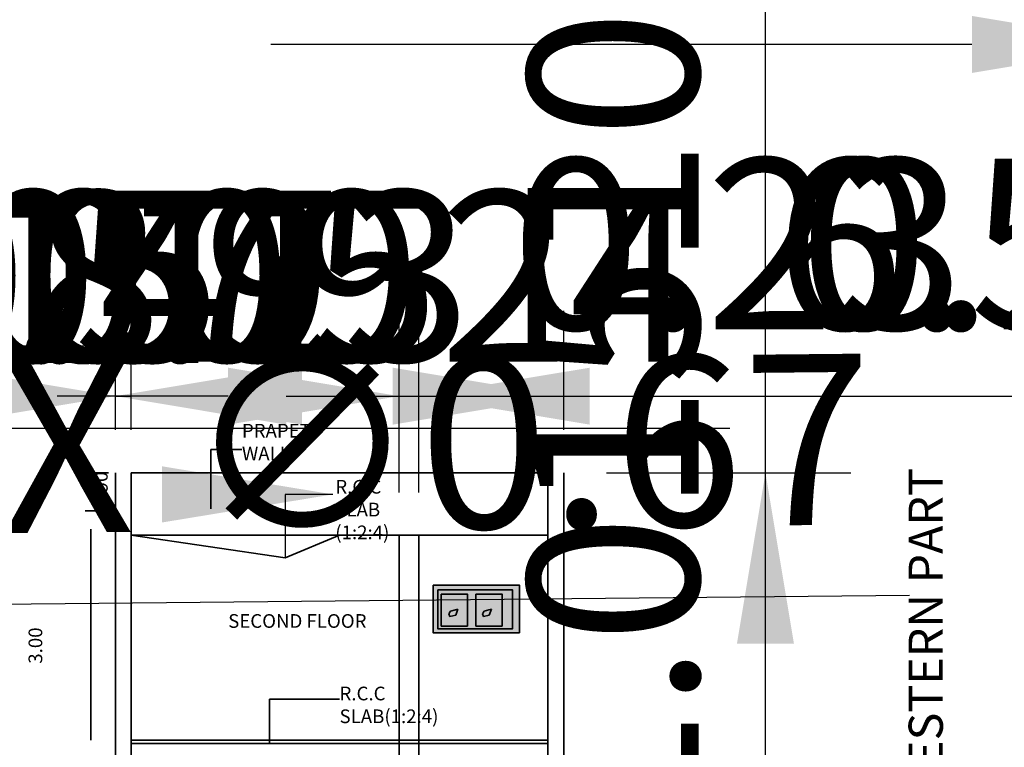
# Model space of a CAD drawing. Units: metres. Extents: x 782 to 1487, y 1262 to 7446.
# Tile 21 of 25: x 801.93 to 816.33, y 1326.35 to 1336.99. Entities that reach past the tile are written whole.
import ezdxf

# ---------------------------------------------------------------- set-up
doc = ezdxf.new("R2010")
doc.units = ezdxf.units.M
for name, color, linetype, lineweight in [('A-ANNO-DIMS', 2, 'Continuous', 18), ('A-ANNO-TEXT', 3, 'Continuous', 18), ('A-SECT', 7, 'Continuous', 35), ('A-SECT-PATT', 9, 'Continuous', 13)]:
    doc.layers.add(name, color=color, linetype=linetype, lineweight=lineweight)
doc.styles.get("Standard").update_dxf_attribs({"font": 'arial.ttf'})
doc.dimstyles.new('ISO-25', dxfattribs={"dimtxt": 2.5, "dimasz": 2.5, "dimexe": 1.25, "dimexo": 0.625, "dimtad": 1, "dimtxsty": 'Standard', "dimcen": 2.5, "dimadec": 0, "dimazin": 0, "dimtfac": 1, "dimtmove": 0, "dimatfit": 3, "dimfxl": 1, "dimarcsym": 0})

# ---------------------------------------------------------------- blocks, each defined once
blk = doc.blocks.new('*D12')
at = {"layer": 'A-ANNO-DIMS', "color": 0, "lineweight": -2, "transparency": 16777216}
for p, q in [((818.357, 1335.252), (818.357, 1337.877)), ((823.837, 1335.252), (823.837, 1337.877)), ((815.857, 1336.627), (805.608, 1336.627)), ((823.837, 1336.627), (818.357, 1336.627)), ((826.337, 1336.627), (828.837, 1336.627))]:
    blk.add_line(p, q, dxfattribs=at)
at = {"layer": 'A-ANNO-DIMS', "color": 0, "transparency": 16777216}
for points in [[(815.857, 1337.044), (815.857, 1336.21), (818.357, 1336.627)], [(826.337, 1337.044), (826.337, 1336.21), (823.837, 1336.627)]]:
    blk.add_solid(points, dxfattribs=at)
at = {"layer": 'Defpoints', "color": 0, "transparency": 16777216}
for p in [(818.357, 1336.627), (818.357, 1334.627), (823.837, 1334.627)]:
    blk.add_point(p, dxfattribs=at)
at = {"layer": 'A-ANNO-DIMS', "color": 0, "transparency": 16777216, "insert": (809.482, 1338.754), "char_height": 2.5, "width": 6.51678, "attachment_point": 5}
blk.add_mtext('5,48', dxfattribs=at)
blk = doc.blocks.new('*D116')
at = {"layer": 'A-ANNO-DIMS', "color": 0, "lineweight": -2, "transparency": 16777216}
for p, q in [((791.782, 1330.988), (791.782, 1332.263)), ((792.923, 1329.614), (792.923, 1332.263)), ((789.282, 1331.013), (786.782, 1331.013)), ((791.782, 1331.013), (792.923, 1331.013)), ((795.423, 1331.013), (805.421, 1331.013))]:
    blk.add_line(p, q, dxfattribs=at)
at = {"layer": 'A-ANNO-DIMS', "color": 0, "transparency": 16777216}
for points in [[(789.282, 1331.43), (789.282, 1330.597), (791.782, 1331.013)], [(795.423, 1331.43), (795.423, 1330.597), (792.923, 1331.013)]]:
    blk.add_solid(points, dxfattribs=at)
at = {"layer": 'Defpoints', "color": 0, "transparency": 16777216}
for p in [(792.923, 1331.013), (791.782, 1330.363), (792.923, 1328.989)]:
    blk.add_point(p, dxfattribs=at)
at = {"layer": 'A-ANNO-DIMS', "color": 0, "transparency": 16777216, "insert": (801.672, 1332.894), "char_height": 2.5, "attachment_point": 5}
blk.add_mtext('1.14', dxfattribs=at)
blk = doc.blocks.new('*D117')
at = {"layer": 'A-ANNO-DIMS', "color": 0, "lineweight": -2, "transparency": 16777216}
for p, q in [((792.923, 1329.614), (792.923, 1332.263)), ((793.726, 1327.207), (793.726, 1332.263)), ((790.423, 1331.013), (787.923, 1331.013)), ((792.923, 1331.013), (793.726, 1331.013)), ((796.226, 1331.013), (806.461, 1331.013))]:
    blk.add_line(p, q, dxfattribs=at)
at = {"layer": 'A-ANNO-DIMS', "color": 0, "transparency": 16777216}
for points in [[(790.423, 1331.43), (790.423, 1330.597), (792.923, 1331.013)], [(796.226, 1331.43), (796.226, 1330.597), (793.726, 1331.013)]]:
    blk.add_solid(points, dxfattribs=at)
at = {"layer": 'Defpoints', "color": 0, "transparency": 16777216}
for p in [(793.726, 1331.013), (792.923, 1328.989), (793.726, 1326.582)]:
    blk.add_point(p, dxfattribs=at)
at = {"layer": 'A-ANNO-DIMS', "color": 0, "transparency": 16777216, "insert": (802.594, 1332.915), "char_height": 2.5, "attachment_point": 5}
blk.add_mtext('0.80', dxfattribs=at)
blk = doc.blocks.new('*D118')
at = {"layer": 'A-ANNO-DIMS', "color": 0, "lineweight": -2, "transparency": 16777216}
for p, q in [((793.726, 1327.207), (793.726, 1332.263)), ((794.32, 1327.207), (794.32, 1332.263)), ((791.226, 1331.013), (788.726, 1331.013)), ((793.726, 1331.013), (794.32, 1331.013)), ((796.82, 1331.013), (807.069, 1331.013))]:
    blk.add_line(p, q, dxfattribs=at)
at = {"layer": 'A-ANNO-DIMS', "color": 0, "transparency": 16777216}
for points in [[(791.226, 1331.43), (791.226, 1330.597), (793.726, 1331.013)], [(796.82, 1331.43), (796.82, 1330.597), (794.32, 1331.013)]]:
    blk.add_solid(points, dxfattribs=at)
at = {"layer": 'Defpoints', "color": 0, "transparency": 16777216}
for p in [(794.32, 1331.013), (793.726, 1326.582), (794.32, 1326.582)]:
    blk.add_point(p, dxfattribs=at)
at = {"layer": 'A-ANNO-DIMS', "color": 0, "transparency": 16777216, "insert": (803.194, 1332.915), "char_height": 2.5, "attachment_point": 5}
blk.add_mtext('0.59', dxfattribs=at)
blk = doc.blocks.new('*D119')
at = {"layer": 'A-ANNO-DIMS', "color": 0, "lineweight": -2, "transparency": 16777216}
for p, q in [((794.32, 1327.207), (794.32, 1332.263)), ((794.83, 1330.074), (794.83, 1332.263)), ((791.82, 1331.013), (789.32, 1331.013)), ((794.32, 1331.013), (794.83, 1331.013)), ((797.33, 1331.013), (807.091, 1331.013))]:
    blk.add_line(p, q, dxfattribs=at)
at = {"layer": 'A-ANNO-DIMS', "color": 0, "transparency": 16777216}
for points in [[(791.82, 1331.43), (791.82, 1330.597), (794.32, 1331.013)], [(797.33, 1331.43), (797.33, 1330.597), (794.83, 1331.013)]]:
    blk.add_solid(points, dxfattribs=at)
at = {"layer": 'Defpoints', "color": 0, "transparency": 16777216}
for p in [(794.83, 1331.013), (794.83, 1329.449), (794.32, 1326.582)]:
    blk.add_point(p, dxfattribs=at)
at = {"layer": 'A-ANNO-DIMS', "color": 0, "transparency": 16777216, "insert": (803.46, 1332.915), "char_height": 2.5, "attachment_point": 5}
blk.add_mtext('0.51', dxfattribs=at)
blk = doc.blocks.new('*D120')
at = {"layer": 'A-ANNO-DIMS', "color": 0, "lineweight": -2, "transparency": 16777216}
for p, q in [((794.83, 1330.074), (794.83, 1332.263)), ((795.62, 1329.519), (795.62, 1332.263)), ((792.33, 1331.013), (789.83, 1331.013)), ((794.83, 1331.013), (795.62, 1331.013)), ((798.12, 1331.013), (808.369, 1331.013))]:
    blk.add_line(p, q, dxfattribs=at)
at = {"layer": 'A-ANNO-DIMS', "color": 0, "transparency": 16777216}
for points in [[(792.33, 1331.43), (792.33, 1330.597), (794.83, 1331.013)], [(798.12, 1331.43), (798.12, 1330.597), (795.62, 1331.013)]]:
    blk.add_solid(points, dxfattribs=at)
at = {"layer": 'Defpoints', "color": 0, "transparency": 16777216}
for p in [(795.62, 1331.013), (794.83, 1329.449), (795.62, 1328.894)]:
    blk.add_point(p, dxfattribs=at)
at = {"layer": 'A-ANNO-DIMS', "color": 0, "transparency": 16777216, "insert": (804.495, 1332.915), "char_height": 2.5, "attachment_point": 5}
blk.add_mtext('0.79', dxfattribs=at)
blk = doc.blocks.new('*D121')
at = {"layer": 'A-ANNO-DIMS', "color": 0, "lineweight": -2, "transparency": 16777216}
for p, q in [((795.62, 1329.519), (795.62, 1332.263)), ((796.354, 1329.519), (796.354, 1332.263)), ((793.12, 1331.013), (790.62, 1331.013)), ((795.62, 1331.013), (796.354, 1331.013)), ((798.854, 1331.013), (809.098, 1331.013))]:
    blk.add_line(p, q, dxfattribs=at)
at = {"layer": 'A-ANNO-DIMS', "color": 0, "transparency": 16777216}
for points in [[(793.12, 1331.43), (793.12, 1330.597), (795.62, 1331.013)], [(798.854, 1331.43), (798.854, 1330.597), (796.354, 1331.013)]]:
    blk.add_solid(points, dxfattribs=at)
at = {"layer": 'Defpoints', "color": 0, "transparency": 16777216}
for p in [(796.354, 1331.013), (795.62, 1328.894), (796.354, 1328.894)]:
    blk.add_point(p, dxfattribs=at)
at = {"layer": 'A-ANNO-DIMS', "color": 0, "transparency": 16777216, "insert": (805.226, 1332.916), "char_height": 2.5, "attachment_point": 5}
blk.add_mtext('0.73', dxfattribs=at)
blk = doc.blocks.new('*D122')
at = {"layer": 'A-ANNO-DIMS', "color": 0, "lineweight": -2, "transparency": 16777216}
for p, q in [((796.354, 1329.519), (796.354, 1332.263)), ((797.878, 1330.988), (797.878, 1332.263)), ((793.854, 1331.013), (791.354, 1331.013)), ((796.354, 1331.013), (797.878, 1331.013)), ((800.378, 1331.013), (812.318, 1331.013))]:
    blk.add_line(p, q, dxfattribs=at)
at = {"layer": 'A-ANNO-DIMS', "color": 0, "transparency": 16777216}
for points in [[(793.854, 1331.43), (793.854, 1330.597), (796.354, 1331.013)], [(800.378, 1331.43), (800.378, 1330.597), (797.878, 1331.013)]]:
    blk.add_solid(points, dxfattribs=at)
at = {"layer": 'Defpoints', "color": 0, "transparency": 16777216}
for p in [(797.878, 1331.013), (797.878, 1330.363), (796.354, 1328.894)]:
    blk.add_point(p, dxfattribs=at)
at = {"layer": 'A-ANNO-DIMS', "color": 0, "transparency": 16777216, "insert": (807.598, 1332.915), "char_height": 2.5, "attachment_point": 5}
blk.add_mtext('1.524', dxfattribs=at)
blk = doc.blocks.new('*D137')
at = {"layer": 'A-ANNO-DIMS', "color": 0, "lineweight": -2, "transparency": 16777216}
for p, q in [((803.332, 1330.988), (803.332, 1332.733)), ((809.888, 1330.988), (809.888, 1332.733)), ((805.832, 1331.483), (807.388, 1331.483)), ((809.888, 1331.483), (822.086, 1331.483))]:
    blk.add_line(p, q, dxfattribs=at)
at = {"layer": 'A-ANNO-DIMS', "color": 0, "transparency": 16777216}
for points in [[(805.832, 1331.899), (805.832, 1331.066), (803.332, 1331.483)], [(807.388, 1331.899), (807.388, 1331.066), (809.888, 1331.483)]]:
    blk.add_solid(points, dxfattribs=at)
at = {"layer": 'Defpoints', "color": 0, "transparency": 16777216}
for p in [(809.888, 1331.483), (803.332, 1330.363), (809.888, 1330.363)]:
    blk.add_point(p, dxfattribs=at)
at = {"layer": 'A-ANNO-DIMS', "color": 0, "transparency": 16777216, "insert": (817.237, 1333.384), "char_height": 2.5, "attachment_point": 5}
blk.add_mtext('6.556', dxfattribs=at)
blk = doc.blocks.new('*D138')
at = {"layer": 'A-ANNO-DIMS', "color": 0, "lineweight": -2, "transparency": 16777216}
for p, q in [((803.332, 1330.988), (803.332, 1332.733)), ((803.562, 1330.988), (803.562, 1332.733)), ((800.832, 1331.483), (798.332, 1331.483)), ((803.332, 1331.483), (803.562, 1331.483)), ((806.062, 1331.483), (816.306, 1331.483))]:
    blk.add_line(p, q, dxfattribs=at)
at = {"layer": 'A-ANNO-DIMS', "color": 0, "transparency": 16777216}
for points in [[(800.832, 1331.899), (800.832, 1331.066), (803.332, 1331.483)], [(806.062, 1331.899), (806.062, 1331.066), (803.562, 1331.483)]]:
    blk.add_solid(points, dxfattribs=at)
at = {"layer": 'Defpoints', "color": 0, "transparency": 16777216}
for p in [(803.562, 1331.483), (803.332, 1330.363), (803.562, 1330.363)]:
    blk.add_point(p, dxfattribs=at)
at = {"layer": 'A-ANNO-DIMS', "color": 0, "transparency": 16777216, "insert": (812.434, 1333.385), "char_height": 2.5, "attachment_point": 5}
blk.add_mtext('0.23', dxfattribs=at)
blk = doc.blocks.new('*D139')
at = {"layer": 'A-ANNO-DIMS', "color": 0, "lineweight": -2, "transparency": 16777216}
for p, q in [((807.481, 1330.074), (807.481, 1332.733)), ((807.769, 1330.074), (807.769, 1332.733)), ((804.981, 1331.483), (802.481, 1331.483)), ((807.481, 1331.483), (807.769, 1331.483)), ((810.269, 1331.483), (820.518, 1331.483))]:
    blk.add_line(p, q, dxfattribs=at)
at = {"layer": 'A-ANNO-DIMS', "color": 0, "transparency": 16777216}
for points in [[(804.981, 1331.899), (804.981, 1331.066), (807.481, 1331.483)], [(810.269, 1331.899), (810.269, 1331.066), (807.769, 1331.483)]]:
    blk.add_solid(points, dxfattribs=at)
at = {"layer": 'Defpoints', "color": 0, "transparency": 16777216}
for p in [(807.769, 1331.483), (807.481, 1329.449), (807.769, 1329.449)]:
    blk.add_point(p, dxfattribs=at)
at = {"layer": 'A-ANNO-DIMS', "color": 0, "transparency": 16777216, "insert": (816.644, 1333.384), "char_height": 2.5, "attachment_point": 5}
blk.add_mtext('0.29', dxfattribs=at)
blk = doc.blocks.new('*D145')
at = {"layer": 'A-ANNO-DIMS', "color": 0, "lineweight": -2, "transparency": 16777216}
for p, q in [((812.839, 1322.045), (812.839, 1334.015)), ((811.308, 1319.545), (814.089, 1319.545)), ((812.839, 1318.53), (812.839, 1319.545)), ((811.308, 1318.53), (814.089, 1318.53)), ((812.839, 1316.03), (812.839, 1313.53))]:
    blk.add_line(p, q, dxfattribs=at)
at = {"layer": 'A-ANNO-DIMS', "color": 0, "transparency": 16777216}
for points in [[(812.422, 1322.045), (813.255, 1322.045), (812.839, 1319.545)], [(812.422, 1316.03), (813.255, 1316.03), (812.839, 1318.53)]]:
    blk.add_solid(points, dxfattribs=at)
at = {"layer": 'Defpoints', "color": 0, "transparency": 16777216}
for p in [(810.683, 1319.545), (812.839, 1319.545), (810.683, 1318.53)]:
    blk.add_point(p, dxfattribs=at)
at = {"layer": 'A-ANNO-DIMS', "color": 0, "transparency": 16777216, "insert": (810.937, 1329.28), "char_height": 2.5, "attachment_point": 5, "rotation": 90}
blk.add_mtext('1.015', dxfattribs=at)
blk = doc.blocks.new('*D146')
at = {"layer": 'A-ANNO-DIMS', "color": 0, "lineweight": -2, "transparency": 16777216}
for p, q in [((812.839, 1330.363), (812.839, 1344.262)), ((810.513, 1330.363), (814.089, 1330.363)), ((812.839, 1322.045), (812.839, 1327.863)), ((810.513, 1319.545), (814.089, 1319.545))]:
    blk.add_line(p, q, dxfattribs=at)
at = {"layer": 'A-ANNO-DIMS', "color": 0, "transparency": 16777216}
for points in [[(812.422, 1327.863), (813.255, 1327.863), (812.839, 1330.363)], [(812.422, 1322.045), (813.255, 1322.045), (812.839, 1319.545)]]:
    blk.add_solid(points, dxfattribs=at)
at = {"layer": 'Defpoints', "color": 0, "transparency": 16777216}
for p in [(809.888, 1330.363), (812.839, 1330.363), (809.888, 1319.545)]:
    blk.add_point(p, dxfattribs=at)
at = {"layer": 'A-ANNO-DIMS', "color": 0, "transparency": 16777216, "insert": (810.937, 1338.563), "char_height": 2.5, "attachment_point": 5, "rotation": 90}
blk.add_mtext('10.818', dxfattribs=at)
blk = doc.blocks.new('*D170')
at = {"layer": 'A-ANNO-DIMS', "color": 0, "lineweight": -2, "transparency": 16777216}
for p, q in [((814.947, 1328.566), (796.747, 1328.385)), ((791.077, 1328.328), (788.578, 1328.304)), ((793.577, 1328.353), (794.248, 1328.36))]:
    blk.add_line(p, q, dxfattribs=at)
at = {"layer": 'A-ANNO-DIMS', "color": 0, "transparency": 16777216}
for points in [[(791.073, 1328.745), (791.082, 1327.912), (793.577, 1328.353)], [(796.743, 1328.802), (796.752, 1327.968), (794.248, 1328.36)]]:
    blk.add_solid(points, dxfattribs=at)
at = {"layer": 'Defpoints', "color": 0, "transparency": 16777216}
for p in [(793.577, 1328.353), (794.248, 1328.36)]:
    blk.add_point(p, dxfattribs=at)
at = {"layer": 'A-ANNO-DIMS', "color": 0, "transparency": 16777216, "insert": (807.078, 1330.459), "char_height": 2.5, "attachment_point": 5, "rotation": 0.5708}
blk.add_mtext('3X ∅0.67', dxfattribs=at)

msp = doc.modelspace()

# ---------------------------------------------------------------- hatches: boundary and pattern name
at = {"layer": 'A-SECT-PATT'}
h = msp.add_hatch(color=256, dxfattribs=at)
h.dxf.hatch_style = 1
h.paths.add_polyline_path([(809.2411, 1328.7199), (807.9777, 1328.7199), (807.9777, 1328.0213), (809.2411, 1328.0213)])
h.paths.add_polyline_path([(809.1376, 1328.0792), (808.0486, 1328.0792), (808.0486, 1328.6511), (809.1376, 1328.6511)], flags=16)
h.paths.add_polyline_path([(808.9875, 1328.1205), (808.6043, 1328.1205), (808.6043, 1328.5874), (808.9875, 1328.5874)], flags=0)
h.paths.add_polyline_path([(808.4803, 1328.1205), (808.0971, 1328.1205), (808.0971, 1328.5874), (808.4803, 1328.5874)], flags=0)
h = msp.add_hatch(color=256, dxfattribs=at)
h.dxf.hatch_style = 1
h.paths.add_polyline_path([(809.1376, 1328.6511), (808.0486, 1328.6511), (808.0486, 1328.0792), (809.1376, 1328.0792)])
h.paths.add_polyline_path([(808.4803, 1328.5874), (808.4803, 1328.1205), (808.0971, 1328.1205), (808.0971, 1328.5874)], flags=16)
h.paths.add_polyline_path([(808.3426, 1328.3672), (808.3106, 1328.2799), (808.224, 1328.2583), (808.2108, 1328.2968), (808.2343, 1328.3373), (808.3059, 1328.357)], flags=0)
h.paths.add_polyline_path([(808.6043, 1328.5874), (808.9875, 1328.5874), (808.9875, 1328.1205), (808.6043, 1328.1205)], flags=16)
h.paths.add_polyline_path([(808.7238, 1328.3373), (808.7953, 1328.357), (808.8321, 1328.3672), (808.8, 1328.2799), (808.7134, 1328.2583), (808.7002, 1328.2968)], flags=0)
h = msp.add_hatch(color=256, dxfattribs=at)
h.dxf.hatch_style = 1
h.paths.add_polyline_path([(808.4803, 1328.5874), (808.0971, 1328.5874), (808.0971, 1328.1205), (808.4803, 1328.1205)])
h.paths.add_polyline_path([(808.3106, 1328.2799), (808.224, 1328.2583), (808.2108, 1328.2968), (808.2343, 1328.3373), (808.3059, 1328.357), (808.3426, 1328.3672)], flags=16)
h.paths.add_polyline_path([(808.9875, 1328.5874), (808.6043, 1328.5874), (808.6043, 1328.1205), (808.9875, 1328.1205)])
h.paths.add_polyline_path([(808.7238, 1328.3373), (808.7953, 1328.357), (808.8321, 1328.3672), (808.8, 1328.2799), (808.7134, 1328.2583), (808.7002, 1328.2968)], flags=16)
h = msp.add_hatch(color=256, dxfattribs=at)
h.dxf.hatch_style = 1
h.paths.add_polyline_path([(808.3426, 1328.3672), (808.3059, 1328.357), (808.2343, 1328.3373), (808.2108, 1328.2968), (808.224, 1328.2583), (808.3106, 1328.2799)])
h.paths.add_polyline_path([(808.8321, 1328.3672), (808.7953, 1328.357), (808.7238, 1328.3373), (808.7002, 1328.2968), (808.7134, 1328.2583), (808.8, 1328.2799)])

# ---------------------------------------------------------------- linework, layer by layer
at = {"layer": 'A-SECT'}
for p, q in [((805.1827, 1330.7028), (804.7268, 1330.7028)), ((804.7268, 1330.7028), (804.7268, 1329.8359)), ((802.8929, 1330.3635), (803.233, 1330.3635)), ((803.3321, 1320.4591), (803.3321, 1330.3635)), ((803.5621, 1330.3635), (809.6581, 1330.3635)), ((803.5621, 1320.4591), (803.5621, 1330.3635)), ((809.6581, 1320.4591), (809.6581, 1330.3635)), ((809.8881, 1320.4591), (809.8881, 1330.3635)), ((803.2609, 1329.8066), (802.8929, 1329.8066)), ((802.9742, 1326.4523), (802.9742, 1329.5361)), ((803.5621, 1329.4495), (809.6581, 1329.4495)), ((805.8175, 1329.1172), (803.5621, 1329.4495)), ((805.8175, 1329.1172), (806.6101, 1329.4495)), ((806.6101, 1329.4495), (805.8175, 1329.1172)), ((807.4812, 1320.4591), (807.4812, 1329.4495)), ((807.7695, 1320.4591), (807.7695, 1329.4495)), ((808.2108, 1328.2968), (808.2343, 1328.3373)), ((808.224, 1328.2583), (808.2108, 1328.2968)), ((808.3106, 1328.2799), (808.224, 1328.2583)), ((808.2343, 1328.3373), (808.3059, 1328.357)), ((808.3059, 1328.357), (808.3426, 1328.3672)), ((808.3426, 1328.3672), (808.3106, 1328.2799)), ((808.7002, 1328.2968), (808.7238, 1328.3373)), ((808.7134, 1328.2583), (808.7002, 1328.2968)), ((808.8, 1328.2799), (808.7134, 1328.2583)), ((808.7238, 1328.3373), (808.7953, 1328.357)), ((808.7953, 1328.357), (808.8321, 1328.3672)), ((808.8321, 1328.3672), (808.8, 1328.2799)), ((805.5843, 1326.4015), (805.5843, 1327.0483)), ((805.5843, 1327.0483), (806.6101, 1327.0483)), ((803.5621, 1326.4523), (809.6581, 1326.4523)), ((803.5621, 1326.4015), (809.6581, 1326.4015)), ((806.6101, 1326.4015), (805.5843, 1326.4015))]:
    msp.add_line(p, q, dxfattribs=at)
for points in [[(807.9777, 1328.7199), (809.2411, 1328.7199), (809.2411, 1328.0213), (807.9777, 1328.0213)], [(808.0486, 1328.6511), (809.1376, 1328.6511), (809.1376, 1328.0792), (808.0486, 1328.0792)], [(808.0971, 1328.5874), (808.4803, 1328.5874), (808.4803, 1328.1205), (808.0971, 1328.1205)], [(808.6043, 1328.5874), (808.9875, 1328.5874), (808.9875, 1328.1205), (808.6043, 1328.1205)]]:
    msp.add_lwpolyline(points, close=True, dxfattribs=at)

# ---------------------------------------------------------------- texts
at = {"layer": 'A-ANNO-TEXT', "char_height": 0.2, "attachment_point": 1}
for s, width, insert in [('\\P\\PPRAPET WALL ', 1.427343, (805.1827, 1331.7444)), ('\\P\\PR.C.C SLAB (1:2:4)', 1.016389, (806.5485, 1330.9238)), ('\\PSECOND FLOOR', 3.104755, (804.9819, 1328.6275)), ('\\PR.C.C SLAB(1:2:4)', 1.857201, (806.6101, 1327.5668))]:
    msp.add_mtext_dynamic_manual_height_columns(s, width=width, gutter_width=12.5, heights=[0], dxfattribs=dict(at, insert=insert))
at = {"layer": 'A-ANNO-TEXT', "attachment_point": 1, "rotation": 90}
for s, width, insert, char_height in [('PLOT NO 127 WESTERN PART', 13.280177, (814.9325, 1321.1357), 0.5), ('\\P0.90', 0.796716, (802.6864, 1329.8478), 0.2), ('3.00', 0.796716, (802.0631, 1327.5694), 0.2)]:
    msp.add_mtext_dynamic_manual_height_columns(s, width=width, gutter_width=12.5, heights=[0], dxfattribs=dict(at, insert=insert, char_height=char_height))

# ---------------------------------------------------------------- dimensions: what is measured, and where the dimension line sits
at = {"layer": 'A-ANNO-DIMS'}
for base, p1, p2, picture, middle in [((812.8387, 1330.3635), (809.8881, 1319.5451), (809.8881, 1330.3635), '*D146', (810.9373, 1338.5627)), ((812.8387, 1319.5451), (810.6826, 1318.53), (810.6826, 1319.5451), '*D145', (810.9373, 1329.2799))]:
    dim = msp.add_linear_dim(base=base, p1=p1, p2=p2, angle=90, dimstyle='ISO-25', override={"dimdec": 3, "dimlfac": 1, "dimrnd": 0, "dimzin": 0, "dimdsep": 46, "dimlunit": 2}, dxfattribs=at)
    dim.commit()
    dim.dimension.update_dxf_attribs({"geometry": picture, "text_midpoint": middle})
for base, p1, p2, override, picture, middle in [((818.357, 1336.627), (823.837, 1334.627), (818.357, 1334.627), {"dimclrd": 0, "dimclre": 0, "dimclrt": 0}, '*D12', (809.4825, 1338.7544)), ((803.5621, 1331.4828), (803.3321, 1330.3635), (803.5621, 1330.3635), {"dimdec": 2, "dimlfac": 1, "dimrnd": 0, "dimzin": 0, "dimdsep": 46, "dimlunit": 2}, '*D138', (812.434, 1333.3851)), ((807.7695, 1331.4828), (807.4812, 1329.4495), (807.7695, 1329.4495), {"dimdec": 2, "dimlfac": 1, "dimrnd": 0, "dimzin": 0, "dimdsep": 46, "dimlunit": 2}, '*D139', (816.6439, 1333.3843)), ((809.8881, 1331.4828), (803.3321, 1330.3635), (809.8881, 1330.3635), {"dimdec": 3, "dimlfac": 1, "dimrnd": 0, "dimzin": 0, "dimdsep": 46, "dimlunit": 2}, '*D137', (817.2371, 1333.3843)), ((792.9231, 1331.0135), (791.7818, 1330.3635), (792.9231, 1328.9889), {"dimdec": 2, "dimlfac": 1, "dimrnd": 0, "dimzin": 0, "dimdsep": 46, "dimlunit": 2}, '*D116', (801.6723, 1332.8936)), ((793.726, 1331.0135), (792.9231, 1328.9889), (793.726, 1326.5822), {"dimdec": 2, "dimlfac": 1, "dimrnd": 0, "dimzin": 0, "dimdsep": 46, "dimlunit": 2}, '*D117', (802.5937, 1332.9149)), ((794.3198, 1331.0135), (793.726, 1326.5822), (794.3198, 1326.5822), {"dimdec": 2, "dimlfac": 1, "dimrnd": 0, "dimzin": 0, "dimdsep": 46, "dimlunit": 2}, '*D118', (803.1943, 1332.9149)), ((794.8298, 1331.0135), (794.3198, 1326.5822), (794.8298, 1329.4495), {"dimdec": 2, "dimlfac": 1, "dimrnd": 0, "dimzin": 0, "dimdsep": 46, "dimlunit": 2}, '*D119', (803.4604, 1332.9149)), ((795.6204, 1331.0135), (794.8298, 1329.4495), (795.6204, 1328.8937), {"dimdec": 2, "dimlfac": 1, "dimrnd": 0, "dimzin": 0, "dimdsep": 46, "dimlunit": 2}, '*D120', (804.4949, 1332.9149)), ((796.3538, 1331.0135), (795.6204, 1328.8937), (796.3538, 1328.8937), {"dimdec": 2, "dimlfac": 1, "dimrnd": 0, "dimzin": 0, "dimdsep": 46, "dimlunit": 2}, '*D121', (805.2257, 1332.9158)), ((797.8778, 1331.0135), (796.3538, 1328.8937), (797.8778, 1330.3635), {"dimdec": 3, "dimlfac": 1, "dimrnd": 0, "dimzin": 0, "dimdsep": 46, "dimlunit": 2}, '*D122', (807.5981, 1332.9149))]:
    dim = msp.add_linear_dim(base=base, p1=p1, p2=p2, dimstyle='ISO-25', override=override, dxfattribs=at)
    dim.commit()
    dim.dimension.update_dxf_attribs({"geometry": picture, "text_midpoint": middle})
dim = msp.add_diameter_dim_2p(p1=(793.5773, 1328.3534), p2=(794.2475, 1328.36), text='3X <>', dimstyle='ISO-25', override={"dimdec": 2, "dimlfac": 1, "dimrnd": 0, "dimzin": 0, "dimdsep": 46, "dimlunit": 2}, dxfattribs=at)
dim.commit()
dim.dimension.update_dxf_attribs({"geometry": '*D170', "text_midpoint": (807.0973, 1328.4881)})

# ---------------------------------------------------------------- leaders
msp.add_leader([(806.5145, 1330.0457), (805.8175, 1330.0457), (805.8175, 1329.1172)], dimstyle='ISO-25', override={"dimgap": 0.625, "dimtad": 0}, dxfattribs=at)

doc.saveas('drawing.dxf')
